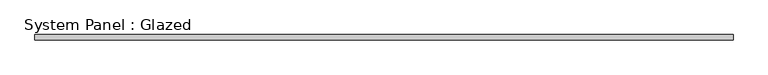
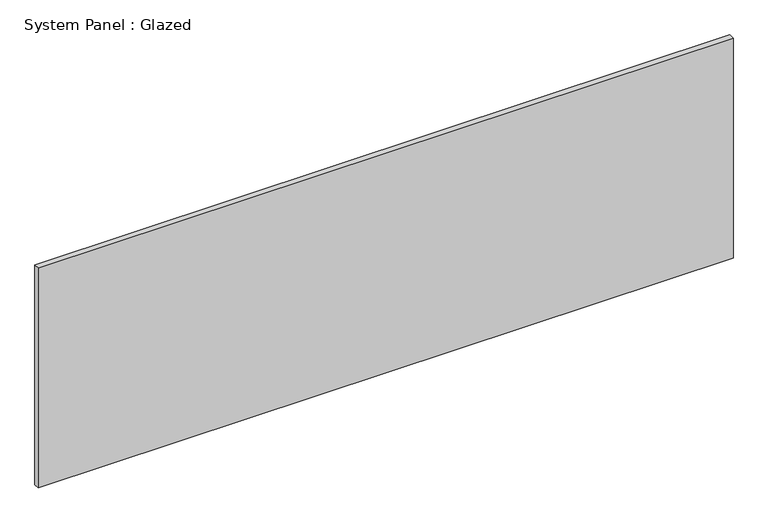
"""IFC4 building model written with IfcOpenShell, lengths in millimetres: plate geometry, System Panel : Glazed."""

from ifc_helpers import new_model, si_unit, origin, origin_with_axes, place, context, project, spatial, polyline, outline, extrude, source, transform, mapped, element, save


def system_panel_glazed_df7f3c5e(model_context):
    return source(origin(), model_context, "Body", "SweptSolid", [
        extrude(outline(polyline([(1631.95, 19.05), (-1631.95, 19.05), (-1631.95, 44.45), (1631.95, 44.45), (1631.95, 19.05)])), origin_with_axes(), (0.0, 0.0, 1.0), 1092.2),
    ])


if __name__ == "__main__":
    model = new_model("IFC4")
    model_context = context("Model", 3, world=origin())
    ifc_project = project(units=[si_unit("LENGTHUNIT", "METRE", prefix="MILLI")], contexts=[model_context])
    site = spatial("IfcSite", under=ifc_project)
    building = spatial("IfcBuilding", under=site)
    placement = place(None, origin())
    system_panel_glazed_shape = system_panel_glazed_df7f3c5e(model_context)
    element("IfcPlate", 1, ObjectType="System Panel : Glazed", at=placement, inside=building, context=model_context, shape_type="MappedRepresentation", body=[
        mapped(system_panel_glazed_shape, transform((0.0, 0.0, 0.0), x_axis=(1.0, 0.0, 0.0), y_axis=(0.0, 1.0, 0.0), z_axis=(0.0, 0.0, 1.0))),
    ])
    save(model, "model.ifc")

# Revit data of these elements
# Type "System Panel : Glazed"
#   Construction Type Id = "GSP4R"
#   Analytic Construction = "1/8 in Pilkington single glazing"
#   Visual Light Transmittance = 0.9
#   Solar Heat Gain Coefficient = 0.86
#   Heat Transfer Coefficient (U) = 1.18115 BTU/(h·ft²·°F)
# Element 1 (IfcPlate, "System Panel : Glazed")
#   Materials on its faces: "Glass"
# Materials
#   "Glass": class "Glass", colour RGB 0 128 192, transparency 0.75, Description = "Soda Lime Glass", Cost = 0
